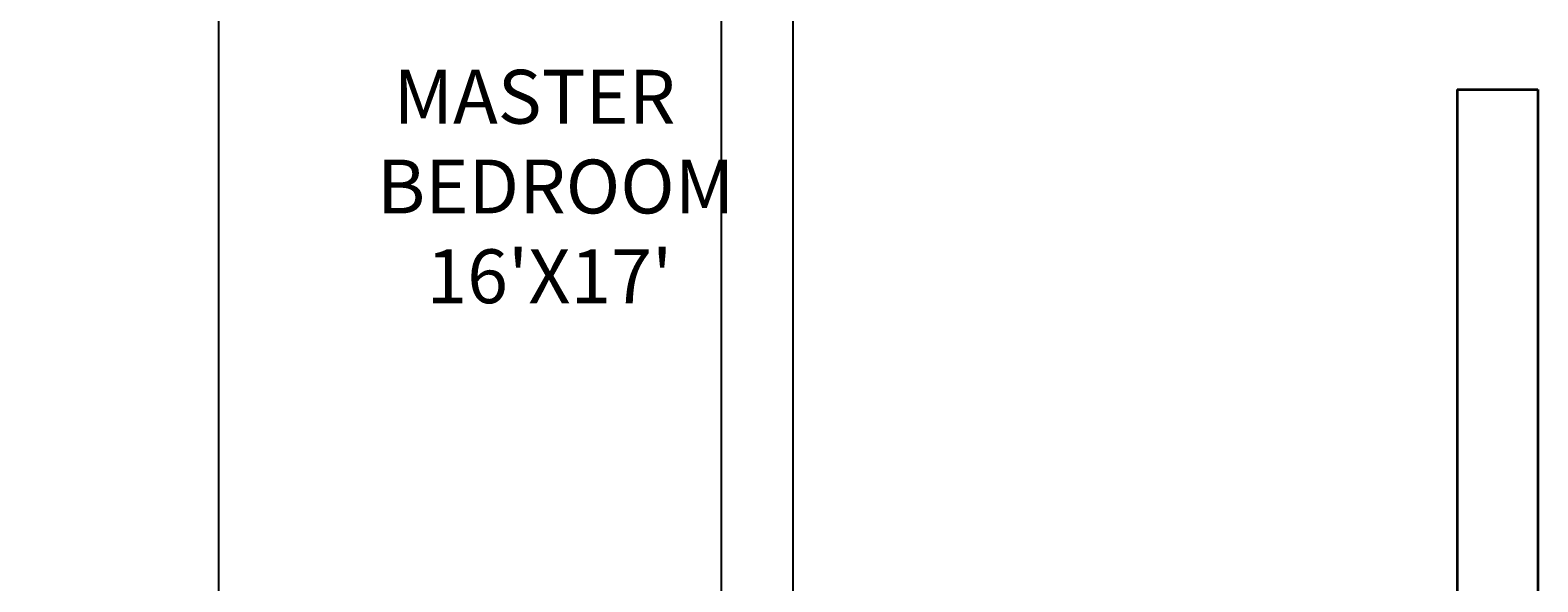
# Model space of a CAD drawing. Units: inches. Extents: x 318 to 927, y -1130 to 13.
# Tile 5 of 17: x 431 to 599, y -929 to -867. Entities that reach past the tile are written whole.
import ezdxf

# ---------------------------------------------------------------- set-up
doc = ezdxf.new("R2010")
doc.units = ezdxf.units.IN
doc.header["$MEASUREMENT"] = 0
for name, color, linetype, lineweight in [('A-ANNO-DIMS', 1, 'Continuous', 18), ('A-AREA-IDEN', 8, 'Continuous', 18), ('wall', 1, 'Continuous', 35)]:
    doc.layers.add(name, color=color, linetype=linetype, lineweight=lineweight)
doc.styles.get("Standard").update_dxf_attribs({"font": 'arial.ttf'})
doc.dimstyles.get("Standard").update_dxf_attribs({"dimtxt": 0.18, "dimasz": 0.18, "dimexe": 0.18, "dimexo": 0.0625, "dimgap": 0.09, "dimtad": 0, "dimtih": 1, "dimtoh": 1, "dimdec": 1, "dimzin": 0, "dimdsep": 46, "dimlunit": 4, "dimtxsty": 'Standard', "dimcen": 0.09, "dimadec": 0, "dimazin": 0, "dimtfac": 1, "dimtdec": 1, "dimtofl": 0, "dimtmove": 0, "dimatfit": 3, "dimfxl": 1, "dimtolj": 1, "dimtzin": 0, "dimarcsym": 0})

# ---------------------------------------------------------------- blocks, each defined once
blk = doc.blocks.new('*D35')
at = {"layer": 'A-ANNO-DIMS', "color": 0, "lineweight": -2, "transparency": 16777216}
for p, q in [((397.89, -457.98), (397.89, -1124.59)), ((451.89, -457.98), (451.89, -1124.59)), ((398.07, -1124.41), (424.56, -1124.41)), ((451.71, -1124.41), (425.23, -1124.41))]:
    blk.add_line(p, q, dxfattribs=at)
at = {"layer": 'A-ANNO-DIMS', "color": 0, "transparency": 16777216}
for points in [[(398.07, -1124.38), (398.07, -1124.44), (397.89, -1124.41)], [(451.71, -1124.38), (451.71, -1124.44), (451.89, -1124.41)]]:
    blk.add_solid(points, dxfattribs=at)
at = {"layer": 'Defpoints', "color": 0, "transparency": 16777216}
for p in [(397.89, -457.91), (451.89, -457.91), (451.89, -1124.41)]:
    blk.add_point(p, dxfattribs=at)
at = {"layer": 'A-ANNO-DIMS', "color": 0, "transparency": 16777216, "insert": (424.89, -1124.41), "char_height": 0.18, "attachment_point": 5}
blk.add_mtext('\\A1;4\'-6"', dxfattribs=at)
blk = doc.blocks.new('*D36')
at = {"layer": 'A-ANNO-DIMS', "color": 0, "lineweight": -2, "transparency": 16777216}
for p, q in [((507.89, -457.98), (507.89, -1124.59)), ((515.89, -457.98), (515.89, -1124.59)), ((508.07, -1124.41), (511.57, -1124.41)), ((515.71, -1124.41), (512.22, -1124.41))]:
    blk.add_line(p, q, dxfattribs=at)
at = {"layer": 'A-ANNO-DIMS', "color": 0, "transparency": 16777216}
for points in [[(508.07, -1124.38), (508.07, -1124.44), (507.89, -1124.41)], [(515.71, -1124.38), (515.71, -1124.44), (515.89, -1124.41)]]:
    blk.add_solid(points, dxfattribs=at)
at = {"layer": 'Defpoints', "color": 0, "transparency": 16777216}
for p in [(507.89, -457.91), (515.89, -457.91), (515.89, -1124.41)]:
    blk.add_point(p, dxfattribs=at)
at = {"layer": 'A-ANNO-DIMS', "color": 0, "transparency": 16777216, "insert": (511.89, -1124.41), "char_height": 0.18, "attachment_point": 5}
blk.add_mtext('\\A1;0\'-8"', dxfattribs=at)

msp = doc.modelspace()

# ---------------------------------------------------------------- linework, layer by layer
at = {"layer": 'wall'}
for p, q in [((589.89, -873.91), (598.89, -873.91)), ((589.89, -873.91), (589.89, -1033.91)), ((598.89, -873.91), (598.89, -1033.91))]:
    msp.add_line(p, q, dxfattribs=at)

# ---------------------------------------------------------------- texts
at = {"layer": 'A-AREA-IDEN', "insert": (469.54, -871.72), "char_height": 6, "attachment_point": 1}
msp.add_mtext_dynamic_manual_height_columns(" MASTER BEDROOM\\P   16'X17'", width=45.6749, gutter_width=1, heights=[0], dxfattribs=at)

# ---------------------------------------------------------------- dimensions: what is measured, and where the dimension line sits
at = {"layer": 'A-ANNO-DIMS'}
for base, p1, p2, picture, middle in [((451.89, -1124.41), (397.89, -457.91), (451.89, -457.91), '*D35', (424.89, -1124.41)), ((515.89, -1124.41), (507.89, -457.91), (515.89, -457.91), '*D36', (511.89, -1124.41))]:
    dim = msp.add_linear_dim(base=base, p1=p1, p2=p2, dimstyle='Standard', override={"dimdec": 1, "dimlfac": 1, "dimrnd": 0, "dimzin": 1, "dimdsep": 46, "dimlunit": 4, "dimfrac": 2}, dxfattribs=at)
    dim.commit()
    dim.dimension.update_dxf_attribs({"geometry": picture, "text_midpoint": middle})

doc.saveas('drawing.dxf')
